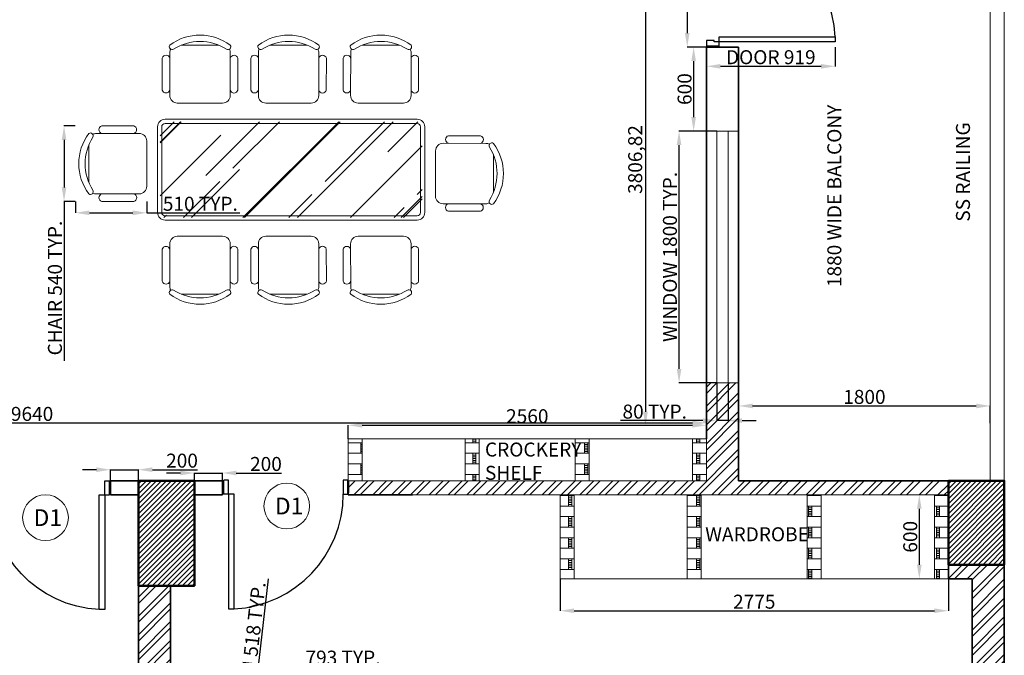
# Model space of a CAD drawing. Units: millimetres. Extents: x -3326 to 29338, y -16792 to 6002.
# Tile 18 of 21: x 22244 to 29282, y -7931 to -3388. Entities that reach past the tile are written whole.
import ezdxf

# ---------------------------------------------------------------- set-up
doc = ezdxf.new("R2010")
doc.units = ezdxf.units.MM
doc.header["$PDMODE"] = 35
doc.header["$PDSIZE"] = 5
for name, color, linetype, lineweight in [('A-ANNO-DIMS', 2, 'Continuous', 13), ('A-ANNO-SYMB', 7, 'Continuous', 18), ('A-AREA-IDEN', 7, 'Continuous', 18), ('A-COLS', 1, 'Continuous', 50), ('A-COLS-PATT', 251, 'Continuous', 13), ('A-DOOR', 3, 'Continuous', 25), ('A-FLOR-CASE', 30, 'Continuous', 18), ('A-FLOR-CASE-PATT', 252, 'Continuous', 13), ('A-FLOR-RAIL', 8, 'Continuous', 20), ('A-FURN-PATT', 252, 'Continuous', 13), ('A-GLAZ', 4, 'Continuous', 18), ('A-WALL', 7, 'Continuous', 35), ('A-WALL-PATT', 252, 'Continuous', 13), ('furn', 28, 'Continuous', 18), ('txt', 7, 'Continuous', 18)]:
    doc.layers.add(name, color=color, linetype=linetype, lineweight=lineweight)
doc.styles.get("Standard").update_dxf_attribs({"font": 'arial.ttf'})
doc.dimstyles.new('ISO-25', dxfattribs={"dimtxt": 100, "dimasz": 100, "dimexe": 1.25, "dimexo": 0.625, "dimtad": 1, "dimtxsty": 'Standard', "dimcen": 2.5, "dimadec": 0, "dimazin": 0, "dimtfac": 1, "dimtmove": 0, "dimatfit": 3, "dimfxl": 1, "dimarcsym": 0})
pattern_1 = [(0, (-10476.645, 1e-12), (0, 75.438), []), (90, (-10270.9, 1e-12), (-114.3, 75.438), [75.438, -75.438]), (90, (-10293.77, 1e-12), (-114.3, 75.438), [75.438, -75.438]), (0, (-10270.905, 12.57), (114.3, 75.438), [-205.74, 22.86]), (0, (-10270.905, 25.146), (114.3, 75.438), [-205.74, 22.86]), (0, (-10270.905, 37.72), (114.3, 75.438), [-205.74, 22.86]), (0, (-10270.905, 50.29), (114.3, 75.438), [-205.74, 22.86]), (0, (-10270.905, 62.865), (114.3, 75.438), [-205.74, 22.86])]
pattern_2 = [(45, (-10476.65, 1e-12), (-67.35192, 67.35192), []), (45, (-10431.74, 1e-12), (-67.35192, 67.35192), [])]

# ---------------------------------------------------------------- blocks, each defined once
blk = doc.blocks.new('A$C13FC179C')
for points in [[(993.9, 100), (920, 100), (920, 1020), (960, 1020), (960, 100), (960, 60), (947.8, 60), (947.8, 0), (993.9, 0)], [(6.1, 0), (46.1, 0), (46.1, 60), (33.9, 60), (33.9, 100), (6.1, 100)], [(6.1, 100), (6.1, 0)], [(993.9, 100), (993.9, 0)]]:
    blk.add_lwpolyline(points)
for points in [[(0, 10), (6.1, 10), (6.1, 90), (0, 90)], [(993.9, 10), (1000, 10), (1000, 90), (993.9, 90)]]:
    blk.add_lwpolyline(points, close=True)
blk.add_arc((960, 100), 920.9, 92.48955, 180)
blk = doc.blocks.new('A$C0CE462CD')
for p, q in [((860, 100), (860, 0)), ((860, 0), (893.9, 0))]:
    blk.add_line(p, q)
for points in [[(860, 100), (860, 920), (818.4, 920), (818.4, 100)], [(0, 10), (6.1, 10), (6.1, 90), (0, 90)], [(893.9, 10), (900, 10), (900, 90), (893.9, 90)]]:
    blk.add_lwpolyline(points, close=True)
for points in [[(6.1, 0), (40, 0), (40, 100), (6.1, 100)], [(6.1, 100), (6.1, 0)], [(860, 100), (893.9, 100), (893.9, 0)]]:
    blk.add_lwpolyline(points)
blk.add_arc((859.1, 101.9), 819.1, 92.8508, 180.13091)
blk = doc.blocks.new('*D16')
at = {"layer": 'A-ANNO-DIMS', "color": 0, "lineweight": -2, "transparency": 16777216}
for p, q in [((26107.3, -7384.6), (26107.3, -7613.9)), ((28882.3, -7384.6), (28882.3, -7613.9)), ((26207.3, -7612.7), (28782.3, -7612.7))]:
    blk.add_line(p, q, dxfattribs=at)
at = {"layer": 'A-ANNO-DIMS', "color": 0, "transparency": 16777216}
for points in [[(26207.3, -7596), (26207.3, -7629.3), (26107.3, -7612.7)], [(28782.3, -7596), (28782.3, -7629.3), (28882.3, -7612.7)]]:
    blk.add_solid(points, dxfattribs=at)
at = {"layer": 'Defpoints', "color": 0, "transparency": 16777216}
for p in [(26107.3, -7384), (28882.3, -7384), (28882.3, -7612.7)]:
    blk.add_point(p, dxfattribs=at)
at = {"layer": 'A-ANNO-DIMS', "color": 0, "transparency": 16777216, "insert": (27494.8, -7561), "char_height": 100, "attachment_point": 5}
blk.add_mtext('2775', dxfattribs=at)
blk = doc.blocks.new('*D31')
at = {"layer": 'A-ANNO-DIMS', "color": 0, "lineweight": -2, "transparency": 16777216}
for p, q in [((22792.3, -6604.5), (22692.3, -6604.5)), ((22892.3, -6683.3), (22892.3, -6603.3)), ((22892.3, -6604.5), (23092.3, -6604.5)), ((23092.3, -6683.3), (23092.3, -6603.3)), ((23192.3, -6604.5), (23515.9, -6604.5))]:
    blk.add_line(p, q, dxfattribs=at)
at = {"layer": 'A-ANNO-DIMS', "color": 0, "transparency": 16777216}
for points in [[(22792.3, -6587.8), (22792.3, -6621.2), (22892.3, -6604.5)], [(23192.3, -6587.8), (23192.3, -6621.2), (23092.3, -6604.5)]]:
    blk.add_solid(points, dxfattribs=at)
at = {"layer": 'Defpoints', "color": 0, "transparency": 16777216}
for p in [(23092.3, -6604.5), (22892.3, -6684), (23092.3, -6684)]:
    blk.add_point(p, dxfattribs=at)
at = {"layer": 'A-ANNO-DIMS', "color": 0, "transparency": 16777216, "insert": (23404.1, -6552.8), "char_height": 100, "attachment_point": 5}
blk.add_mtext('200', dxfattribs=at)
blk = doc.blocks.new('*D32')
at = {"layer": 'A-ANNO-DIMS', "color": 0, "lineweight": -2, "transparency": 16777216}
for p, q in [((23392.3, -6628.3), (23292.3, -6628.3)), ((23492.3, -6683.3), (23492.3, -6627)), ((23492.3, -6628.3), (23692.3, -6628.3)), ((23692.3, -6683.3), (23692.3, -6627)), ((23792.3, -6628.3), (24115.9, -6628.3))]:
    blk.add_line(p, q, dxfattribs=at)
at = {"layer": 'A-ANNO-DIMS', "color": 0, "transparency": 16777216}
for points in [[(23392.3, -6611.6), (23392.3, -6644.9), (23492.3, -6628.3)], [(23792.3, -6611.6), (23792.3, -6644.9), (23692.3, -6628.3)]]:
    blk.add_solid(points, dxfattribs=at)
at = {"layer": 'Defpoints', "color": 0, "transparency": 16777216}
for p in [(23492.3, -6684), (23692.3, -6628.3), (23692.3, -6684)]:
    blk.add_point(p, dxfattribs=at)
at = {"layer": 'A-ANNO-DIMS', "color": 0, "transparency": 16777216, "insert": (24004.1, -6576.6), "char_height": 100, "attachment_point": 5}
blk.add_mtext('200', dxfattribs=at)
blk = doc.blocks.new('*D33')
at = {"layer": 'A-ANNO-DIMS', "color": 0, "lineweight": -2, "transparency": 16777216}
for p, q in [((24592.3, -6383.3), (24592.3, -6285.8)), ((24692.3, -6287), (27052.3, -6287)), ((27152.3, -6383.3), (27152.3, -6285.8))]:
    blk.add_line(p, q, dxfattribs=at)
at = {"layer": 'A-ANNO-DIMS', "color": 0, "transparency": 16777216}
for points in [[(24692.3, -6270.4), (24692.3, -6303.7), (24592.3, -6287)], [(27052.3, -6270.4), (27052.3, -6303.7), (27152.3, -6287)]]:
    blk.add_solid(points, dxfattribs=at)
at = {"layer": 'Defpoints', "color": 0, "transparency": 16777216}
for p in [(27152.3, -6287), (24592.3, -6384), (27152.3, -6384)]:
    blk.add_point(p, dxfattribs=at)
at = {"layer": 'A-ANNO-DIMS', "color": 0, "transparency": 16777216, "insert": (25872.3, -6235.3), "char_height": 100, "attachment_point": 5}
blk.add_mtext('2560', dxfattribs=at)
blk = doc.blocks.new('*D83')
at = {"layer": 'A-ANNO-DIMS', "color": 0, "lineweight": -2, "transparency": 16777216}
for p, q in [((28675.2, -6784), (28675.9, -6784)), ((28674.6, -6884), (28674.6, -7284)), ((28675.2, -7384), (28675.9, -7384))]:
    blk.add_line(p, q, dxfattribs=at)
at = {"layer": 'A-ANNO-DIMS', "color": 0, "transparency": 16777216}
for points in [[(28657.9, -6884), (28691.3, -6884), (28674.6, -6784)], [(28657.9, -7284), (28691.3, -7284), (28674.6, -7384)]]:
    blk.add_solid(points, dxfattribs=at)
at = {"layer": 'Defpoints', "color": 0, "transparency": 16777216}
for p in [(28674.6, -6784), (28674.6, -7384), (28674.6, -7384)]:
    blk.add_point(p, dxfattribs=at)
at = {"layer": 'A-ANNO-DIMS', "color": 0, "transparency": 16777216, "insert": (28622.9, -7084), "char_height": 100, "attachment_point": 5, "rotation": 90}
blk.add_mtext('600', dxfattribs=at)
blk = doc.blocks.new('*D93')
at = {"layer": 'A-ANNO-DIMS', "color": 0, "lineweight": -2, "transparency": 16777216}
for p, q in [((27382.3, -6273.2), (27382.3, -6147.7)), ((27482.3, -6148.9), (29082.3, -6148.9)), ((29182.3, -6273.2), (29182.3, -6147.7))]:
    blk.add_line(p, q, dxfattribs=at)
at = {"layer": 'A-ANNO-DIMS', "color": 0, "transparency": 16777216}
for points in [[(27482.3, -6132.3), (27482.3, -6165.6), (27382.3, -6148.9)], [(29082.3, -6132.3), (29082.3, -6165.6), (29182.3, -6148.9)]]:
    blk.add_solid(points, dxfattribs=at)
at = {"layer": 'Defpoints', "color": 0, "transparency": 16777216}
for p in [(29182.3, -6148.9), (27382.3, -6273.8), (29182.3, -6273.8)]:
    blk.add_point(p, dxfattribs=at)
at = {"layer": 'A-ANNO-DIMS', "color": 0, "transparency": 16777216, "insert": (28282.3, -6097.3), "char_height": 100, "attachment_point": 5}
blk.add_mtext('1800', dxfattribs=at)
blk = doc.blocks.new('*D94')
at = {"layer": 'A-ANNO-DIMS', "color": 0, "lineweight": -2, "transparency": 16777216}
for p, q in [((27151.7, -3584), (27060.1, -3584)), ((27061.4, -3684), (27061.4, -4084)), ((27151.7, -4184), (27060.1, -4184))]:
    blk.add_line(p, q, dxfattribs=at)
at = {"layer": 'A-ANNO-DIMS', "color": 0, "transparency": 16777216}
for points in [[(27044.7, -3684), (27078.1, -3684), (27061.4, -3584)], [(27044.7, -4084), (27078.1, -4084), (27061.4, -4184)]]:
    blk.add_solid(points, dxfattribs=at)
at = {"layer": 'Defpoints', "color": 0, "transparency": 16777216}
for p in [(27152.3, -3584), (27061.4, -4184), (27152.3, -4184)]:
    blk.add_point(p, dxfattribs=at)
at = {"layer": 'A-ANNO-DIMS', "color": 0, "transparency": 16777216, "insert": (27009.7, -3884), "char_height": 100, "attachment_point": 5, "rotation": 90}
blk.add_mtext('600', dxfattribs=at)
blk = doc.blocks.new('*D96')
at = {"layer": 'A-ANNO-DIMS', "color": 0, "lineweight": -2, "transparency": 16777216}
for p, q in [((26717.8, -2484), (26718.5, -2484)), ((26717.2, -2584), (26717.2, -6190.8)), ((26717.8, -6290.8), (26718.5, -6290.8))]:
    blk.add_line(p, q, dxfattribs=at)
at = {"layer": 'A-ANNO-DIMS', "color": 0, "transparency": 16777216}
for points in [[(26700.5, -2584), (26733.9, -2584), (26717.2, -2484)], [(26700.5, -6190.8), (26733.9, -6190.8), (26717.2, -6290.8)]]:
    blk.add_solid(points, dxfattribs=at)
at = {"layer": 'Defpoints', "color": 0, "transparency": 16777216}
for p in [(26717.2, -2484), (26717.2, -6290.8), (26717.2, -6290.8)]:
    blk.add_point(p, dxfattribs=at)
at = {"layer": 'A-ANNO-DIMS', "color": 0, "transparency": 16777216, "insert": (26656.5, -4387.4), "char_height": 100, "attachment_point": 5, "rotation": 90}
blk.add_mtext('3806,82', dxfattribs=at)
blk = doc.blocks.new('*D97')
at = {"layer": 'A-ANNO-DIMS', "color": 0, "lineweight": -2, "transparency": 16777216}
for p, q in [((27152.3, -6119.9), (27152.3, -6271.6)), ((17512.3, -6265.8), (17512.3, -6271.6)), ((17612.3, -6270.4), (27052.3, -6270.4))]:
    blk.add_line(p, q, dxfattribs=at)
at = {"layer": 'A-ANNO-DIMS', "color": 0, "transparency": 16777216}
for points in [[(17612.3, -6253.7), (17612.3, -6287), (17512.3, -6270.4)], [(27052.3, -6253.7), (27052.3, -6287), (27152.3, -6270.4)]]:
    blk.add_solid(points, dxfattribs=at)
at = {"layer": 'Defpoints', "color": 0, "transparency": 16777216}
for p in [(27152.3, -6119.3), (17512.3, -6265.2), (27152.3, -6270.4)]:
    blk.add_point(p, dxfattribs=at)
at = {"layer": 'A-ANNO-DIMS', "color": 0, "transparency": 16777216, "insert": (22332.3, -6218.7), "char_height": 100, "attachment_point": 5}
blk.add_mtext('9640', dxfattribs=at)
blk = doc.blocks.new('CHAIR-DINING')
for p, q in [((54.3, 125.8), (54, 431.8)), ((107.9, 485.8), (431.9, 486.2)), ((486, 432.2), (486.3, 126.2)), ((0, 393.5), (0.2, 164)), ((540, 394), (540.2, 164.5)), ((404.2, 72.1), (136.4, 71.9))]:
    blk.add_line(p, q)
for centre, radius, start, end in [((108, 431.8), 54, 90.0573, 180.0573), ((432, 432.2), 54, 0.0573, 90.0573), ((27, 385.6), 28.1, 16.3175, 163.79709), ((513, 386.1), 28.1, 16.3175, 163.79709), ((27.2, 171.9), 28.1, 196.3175, 343.79709), ((513.2, 172.4), 28.1, 196.3175, 343.79709), ((70.1, 83.6), 19.7, 58.02988, 216.74736), ((108.3, 125.8), 54, 180.0573, 207.64174), ((270, 360), 360, 233.1874, 306.92719), ((270, 399.2), 353.5, 237.63305, 302.48154), ((470.5, 84), 19.7, 323.36723, 122.08471), ((432.3, 126.2), 54, 332.47286, 0.0573)]:
    blk.add_arc(centre, radius, start, end)
blk = doc.blocks.new('TAG-D1')
blk.add_circle((163.3, 163.3), 163.3)
at = {"insert": (78, 223.5), "char_height": 120, "attachment_point": 1}
blk.add_mtext_dynamic_manual_height_columns('D1', width=137.943, gutter_width=12.5, heights=[0], dxfattribs=at)
blk = doc.blocks.new('GLAZ-1800x80')
for p, q in [((0, 80), (1800, 80)), ((0, 0), (1800, 0))]:
    blk.add_line(p, q)
blk = doc.blocks.new('*D190')
at = {"layer": 'A-ANNO-DIMS', "color": 0, "lineweight": -2, "transparency": 16777216}
for p, q in [((24158.2, -8133.6), (24158.2, -8011.3)), ((24258.2, -8012.6), (24851.6, -8012.6)), ((24951.6, -8133.6), (24951.6, -8011.3))]:
    blk.add_line(p, q, dxfattribs=at)
at = {"layer": 'A-ANNO-DIMS', "color": 0, "transparency": 16777216}
for points in [[(24258.2, -7995.9), (24258.2, -8029.2), (24158.2, -8012.6)], [(24851.6, -7995.9), (24851.6, -8029.2), (24951.6, -8012.6)]]:
    blk.add_solid(points, dxfattribs=at)
at = {"layer": 'Defpoints', "color": 0, "transparency": 16777216}
for p in [(24951.6, -8012.6), (24158.2, -8134.2), (24951.6, -8134.2)]:
    blk.add_point(p, dxfattribs=at)
at = {"layer": 'A-ANNO-DIMS', "color": 0, "transparency": 16777216, "insert": (24554.9, -7960.9), "char_height": 100, "attachment_point": 5}
blk.add_mtext('793 TYP.', dxfattribs=at)
blk = doc.blocks.new('*D201')
at = {"layer": 'A-ANNO-DIMS', "color": 0, "lineweight": -2, "transparency": 16777216}
for p, q in [((27153.3, -3584), (27153.3, -3722.5)), ((28072.8, -3584), (28072.8, -3722.5)), ((27253.3, -3721.3), (27972.8, -3721.3))]:
    blk.add_line(p, q, dxfattribs=at)
at = {"layer": 'A-ANNO-DIMS', "color": 0, "transparency": 16777216}
for points in [[(27253.3, -3704.6), (27253.3, -3737.9), (27153.3, -3721.3)], [(27972.8, -3704.6), (27972.8, -3737.9), (28072.8, -3721.3)]]:
    blk.add_solid(points, dxfattribs=at)
at = {"layer": 'Defpoints', "color": 0, "transparency": 16777216}
for p in [(27153.3, -3583.3), (28072.8, -3583.3), (28072.8, -3721.3)]:
    blk.add_point(p, dxfattribs=at)
at = {"layer": 'A-ANNO-DIMS', "color": 0, "transparency": 16777216, "insert": (27613.1, -3668.9), "char_height": 100, "attachment_point": 5}
blk.add_mtext('DOOR 919', dxfattribs=at)
blk = doc.blocks.new('*D202')
at = {"layer": 'A-ANNO-DIMS', "color": 0, "lineweight": -2, "transparency": 16777216}
for p, q in [((27152.7, -2681.9), (27014.2, -2681.9)), ((27015.4, -2781.9), (27015.4, -3483.3)), ((27152.7, -3583.3), (27014.2, -3583.3))]:
    blk.add_line(p, q, dxfattribs=at)
at = {"layer": 'A-ANNO-DIMS', "color": 0, "transparency": 16777216}
for points in [[(26998.8, -2781.9), (27032.1, -2781.9), (27015.4, -2681.9)], [(26998.8, -3483.3), (27032.1, -3483.3), (27015.4, -3583.3)]]:
    blk.add_solid(points, dxfattribs=at)
at = {"layer": 'Defpoints', "color": 0, "transparency": 16777216}
for p in [(27153.3, -2681.9), (27015.4, -3583.3), (27153.3, -3583.3)]:
    blk.add_point(p, dxfattribs=at)
at = {"layer": 'A-ANNO-DIMS', "color": 0, "transparency": 16777216, "insert": (26963.7, -3132.6), "char_height": 100, "attachment_point": 5, "rotation": 90}
blk.add_mtext('901', dxfattribs=at)
blk = doc.blocks.new('*D203')
at = {"layer": 'A-ANNO-DIMS', "color": 0, "lineweight": -2, "transparency": 16777216}
for p, q in [((27226.7, -4184), (26956.1, -4184)), ((26957.3, -5884), (26957.3, -4284)), ((27226.7, -5984), (26956.1, -5984))]:
    blk.add_line(p, q, dxfattribs=at)
at = {"layer": 'A-ANNO-DIMS', "color": 0, "transparency": 16777216}
for points in [[(26940.6, -4284), (26974, -4284), (26957.3, -4184)], [(26940.6, -5884), (26974, -5884), (26957.3, -5984)]]:
    blk.add_solid(points, dxfattribs=at)
at = {"layer": 'Defpoints', "color": 0, "transparency": 16777216}
for p in [(26957.3, -4184), (27227.3, -4184), (27227.3, -5984)]:
    blk.add_point(p, dxfattribs=at)
at = {"layer": 'A-ANNO-DIMS', "color": 0, "transparency": 16777216, "insert": (26904.9, -5084), "char_height": 100, "attachment_point": 5, "rotation": 90}
blk.add_mtext('WINDOW 1800 TYP.', dxfattribs=at)
blk = doc.blocks.new('*D204')
at = {"layer": 'A-ANNO-DIMS', "color": 0, "lineweight": -2, "transparency": 16777216}
for p, q in [((27227.3, -5984.6), (27227.3, -6255.2)), ((27307.3, -5984.6), (27307.3, -6255.2)), ((27127.3, -6254), (26539.1, -6254)), ((27307.3, -6254), (27227.3, -6254)), ((27407.3, -6254), (27507.3, -6254))]:
    blk.add_line(p, q, dxfattribs=at)
at = {"layer": 'A-ANNO-DIMS', "color": 0, "transparency": 16777216}
for points in [[(27127.3, -6237.3), (27127.3, -6270.6), (27227.3, -6254)], [(27407.3, -6237.3), (27407.3, -6270.6), (27307.3, -6254)]]:
    blk.add_solid(points, dxfattribs=at)
at = {"layer": 'Defpoints', "color": 0, "transparency": 16777216}
for p in [(27227.3, -5984), (27307.3, -5984), (27227.3, -6254)]:
    blk.add_point(p, dxfattribs=at)
at = {"layer": 'A-ANNO-DIMS', "color": 0, "transparency": 16777216, "insert": (26783.2, -6202.3), "char_height": 100, "attachment_point": 5}
blk.add_mtext('80 TYP.', dxfattribs=at)
blk = doc.blocks.new('*D211')
at = {"layer": 'A-ANNO-DIMS', "color": 0, "lineweight": -2, "transparency": 16777216}
for p, q in [((22641.2, -4147.1), (22559.6, -4147.1)), ((22560.8, -4247.1), (22560.8, -4587.3)), ((22641.2, -4687.3), (22559.6, -4687.3)), ((22560.8, -4687.3), (22560.8, -5825.4))]:
    blk.add_line(p, q, dxfattribs=at)
at = {"layer": 'A-ANNO-DIMS', "color": 0, "transparency": 16777216}
for points in [[(22544.2, -4247.1), (22577.5, -4247.1), (22560.8, -4147.1)], [(22544.2, -4587.3), (22577.5, -4587.3), (22560.8, -4687.3)]]:
    blk.add_solid(points, dxfattribs=at)
at = {"layer": 'Defpoints', "color": 0, "transparency": 16777216}
for p in [(22641.9, -4147.1), (22560.8, -4687.3), (22641.9, -4687.3)]:
    blk.add_point(p, dxfattribs=at)
at = {"layer": 'A-ANNO-DIMS', "color": 0, "transparency": 16777216, "insert": (22508.5, -5306.4), "char_height": 100, "attachment_point": 5, "rotation": 90}
blk.add_mtext('CHAIR 540 TYP.', dxfattribs=at)
blk = doc.blocks.new('*D212')
at = {"layer": 'A-ANNO-DIMS', "color": 0, "lineweight": -2, "transparency": 16777216}
for p, q in [((22641.9, -4688), (22641.9, -4769.6)), ((23152.1, -4688), (23152.1, -4769.6)), ((22741.9, -4768.4), (23052.1, -4768.4)), ((23152.1, -4768.4), (23817.8, -4768.4))]:
    blk.add_line(p, q, dxfattribs=at)
at = {"layer": 'A-ANNO-DIMS', "color": 0, "transparency": 16777216}
for points in [[(22741.9, -4751.7), (22741.9, -4785), (22641.9, -4768.4)], [(23052.1, -4751.7), (23052.1, -4785), (23152.1, -4768.4)]]:
    blk.add_solid(points, dxfattribs=at)
at = {"layer": 'Defpoints', "color": 0, "transparency": 16777216}
for p in [(22641.9, -4687.3), (23152.1, -4687.3), (23152.1, -4768.4)]:
    blk.add_point(p, dxfattribs=at)
at = {"layer": 'A-ANNO-DIMS', "color": 0, "transparency": 16777216, "insert": (23535, -4716.7), "char_height": 100, "attachment_point": 5}
blk.add_mtext('510 TYP.', dxfattribs=at)
blk = doc.blocks.new('*D215')
at = {"layer": 'A-ANNO-DIMS', "color": 0, "lineweight": -2, "transparency": 16777216}
for p, q in [((23896.1, -8496.3), (24021.7, -7384)), ((23819.5, -8487.6), (23897.4, -8496.4)), ((23849.2, -8911.8), (23884.9, -8595.6)), ((23761.4, -9002.6), (23839.2, -9011.3))]:
    blk.add_line(p, q, dxfattribs=at)
at = {"layer": 'A-ANNO-DIMS', "color": 0, "transparency": 16777216}
for points in [[(23868.3, -8593.8), (23901.5, -8597.5), (23896.1, -8496.3)], [(23832.6, -8910), (23865.8, -8913.7), (23838, -9011.2)]]:
    blk.add_solid(points, dxfattribs=at)
at = {"layer": 'Defpoints', "color": 0, "transparency": 16777216}
for p in [(23818.9, -8487.6), (23896.1, -8496.3), (23760.8, -9002.5)]:
    blk.add_point(p, dxfattribs=at)
at = {"layer": 'A-ANNO-DIMS', "color": 0, "transparency": 16777216, "insert": (23912.5, -7884.6), "char_height": 100, "attachment_point": 5, "rotation": 83.55971}
blk.add_mtext('BASIN 518 TYP.', dxfattribs=at)

msp = doc.modelspace()

# ---------------------------------------------------------------- hatches: boundary and pattern name
at = {"layer": 'A-COLS-PATT'}
h = msp.add_hatch(dxfattribs=at)
h.set_pattern_fill('ANSI31', color=256, scale=8)
h.set_pattern_definition([(45, (-18946.33, 3485.585), (-17.960512, 17.960512), [])])
h.paths.add_polyline_path([(23492.301, -6683.952), (23092.301, -6683.952), (23092.301, -7433.952), (23492.301, -7433.952)])
h = msp.add_hatch(dxfattribs=at)
h.set_pattern_fill('ANSI31', color=256, scale=8)
h.set_pattern_definition([(45, (-12839, -76.948), (-17.960512, 17.960512), [])])
h.paths.add_polyline_path([(28882.301, -7283.952), (29282.301, -7283.952), (29282.301, -6683.952), (28882.301, -6683.952)])
at = {"layer": 'A-FLOR-CASE-PATT'}
h = msp.add_hatch(dxfattribs=at)
h.set_pattern_fill('BRSTONE', color=256, scale=9)
h.set_pattern_definition(pattern_1)
h.paths.add_polyline_path([(24692.301, -6383.952), (24592.301, -6383.952), (24592.301, -6683.952), (24692.301, -6683.952)])
h.paths.add_polyline_path([(25528.967, -6383.952), (25428.967, -6383.952), (25428.967, -6683.952), (25528.967, -6683.952)])
h.paths.add_polyline_path([(26315.634, -6383.952), (26215.634, -6383.952), (26215.634, -6683.952), (26315.634, -6683.952)])
h.paths.add_polyline_path([(27152.301, -6383.952), (27052.301, -6383.952), (27052.301, -6683.952), (27152.301, -6683.952)])
h = msp.add_hatch(dxfattribs=at)
h.set_pattern_fill('BRSTONE', color=256, scale=9)
h.set_pattern_definition(pattern_1)
h.paths.add_polyline_path([(26207.301, -6783.952), (26107.301, -6783.952), (26107.301, -7383.952), (26207.301, -7383.952)])
h.paths.add_polyline_path([(27115.634, -6783.952), (27015.634, -6783.952), (27015.634, -7383.952), (27115.634, -7383.952)])
h.paths.add_polyline_path([(27873.967, -7383.952), (27973.967, -7383.952), (27973.967, -6783.952), (27873.967, -6783.952)])
h.paths.add_polyline_path([(28782.301, -7383.952), (28882.301, -7383.952), (28882.301, -7283.952), (28882.301, -6783.952), (28782.301, -6783.952)])
h.paths.add_polyline_path([(27117.498, -7172.598), (27990.213, -7172.598), (27990.213, -6966.527), (27117.498, -6966.527)], flags=9)
at = {"layer": 'A-FURN-PATT'}
h = msp.add_hatch(dxfattribs=at)
h.set_pattern_fill('AR-RROOF', color=256, scale=400, angle=-135, style=0)
h.set_pattern_definition([(225, (64133.74, 17389.84), (-339.4113, -905.0967), [6000, -800, 2000, -400]), (225, (63899, 16872.24), (659.0235, -93.338), [1200, -132, 2400, -300]), (225, (64232.74, 17008), (-1281.2775, -1660.2867), [3200, -560, 1600, -400])])
edge = h.paths.add_edge_path()
edge.add_line((25121.037, -4765.986), (25121.037, -4153.986))
edge.add_arc((25085.037, -4153.986), 36, 0, 90)
edge.add_line((25085.037, -4117.986), (23283.037, -4117.986))
edge.add_arc((23283.037, -4153.986), 36, 90, 180)
edge.add_line((23247.037, -4153.986), (23247.037, -4765.986))
edge.add_arc((23283.037, -4765.986), 36, -180, -90)
edge.add_line((23283.037, -4801.986), (25085.037, -4801.986))
edge.add_arc((25085.037, -4765.986), 36, -90, 0)
at = {"layer": 'A-WALL-PATT'}
h = msp.add_hatch(dxfattribs=at)
h.set_pattern_fill('ANSI32', color=256, scale=10)
h.set_pattern_definition(pattern_2)
h.paths.add_polyline_path([(29282.301, -7283.952), (28882.301, -7283.952), (28882.301, -7383.952), (29052.301, -7383.952), (29052.301, -10763.952), (29282.301, -10763.952)])
h.paths.add_polyline_path([(29282.301, -11263.952), (29052.301, -11263.952), (29052.301, -12763.952), (29282.301, -12763.952)])
h.paths.add_polyline_path([(25052.301, -11263.952), (25652.301, -11263.952), (25652.301, -11123.904), (25652.289, -11123.904), (25652.289, -11033.952), (25052.301, -11033.952), (24572.301, -11033.952), (24572.301, -11263.952), (24822.301, -11263.952), (24822.301, -12763.952), (25052.301, -12763.952)])
h.paths.add_polyline_path([(26902.301, -11033.952), (26552.301, -11033.952), (26552.301, -11263.952), (26902.301, -11263.952)])
h.paths.add_polyline_path([(21992.301, -6683.952), (21362.301, -6683.952), (17512.301, -6683.952), (17512.301, -6783.952), (21362.301, -6783.952), (21992.301, -6783.952)])
h.paths.add_polyline_path([(17512.301, -7283.952), (17282.301, -7283.952), (17282.301, -12163.952), (17512.301, -12163.952), (17512.301, -11263.952), (18112.301, -11263.952), (18112.301, -11033.952), (17512.301, -11033.952)])
h.paths.add_polyline_path([(21462.301, -8211.864), (21462.064, -8211.864), (21462.064, -8142.609), (21462.301, -8133.952), (21362.301, -8133.952), (21362.301, -8233.952), (21362.301, -11033.952), (21162.301, -11033.952), (21162.301, -11263.952), (21362.301, -11263.952), (21362.301, -12763.952), (21592.301, -12763.952), (21592.301, -11263.952), (21992.301, -11263.952), (21992.301, -11033.952), (21592.301, -11033.952), (21462.301, -11033.952)])
h.paths.add_polyline_path([(24152.301, -8133.952), (23322.301, -8133.952), (23322.301, -7433.952), (23092.301, -7433.952), (23092.301, -8133.952), (22241.021, -8133.952), (22241.021, -8142.609), (22241.182, -8142.609), (22241.182, -8211.864), (22241.021, -8233.952), (23092.301, -8233.952), (23092.301, -10513.206), (23322.301, -10513.206), (23322.301, -8233.952), (24152.301, -8233.952)])
h.paths.add_polyline_path([(25052.301, -8233.952), (25052.301, -8133.952), (24952.301, -8133.952), (24952.301, -11033.952), (25052.301, -11033.952)])
h.paths.add_polyline_path([(23972.301, -11033.952), (23493.251, -11033.952), (23493.251, -11263.952), (23972.301, -11263.952)])
h.paths.add_polyline_path([(23092.301, -11033.952), (22592.301, -11033.952), (22592.301, -11263.952), (23092.301, -11263.952)])
h.paths.add_polyline_path([(28882.301, -11033.952), (28702.301, -11033.952), (28702.301, -11263.952), (28882.301, -11263.952)])
h.paths.add_polyline_path([(17512.301, -3883.952), (17387.589, -3883.952), (17387.589, -3888.07), (17282.301, -3888.07), (17282.301, -6683.952), (17512.301, -6683.952)])
h.paths.add_polyline_path([(21462.301, -2183.952), (21362.301, -2183.952), (21362.301, -2383.952), (17282.301, -2383.952), (17282.301, -2483.952), (17512.301, -2483.952), (21462.301, -2483.952)])
h.paths.add_polyline_path([(17512.301, -2483.952), (17282.301, -2483.952), (17282.301, -2833.952), (17512.301, -2833.952)])
h.paths.add_polyline_path([(21462.301, 1866.048), (21992.301, 1866.048), (21992.301, 2096.048), (21592.301, 2096.048), (21592.301, 3596.048), (21362.301, 3596.048), (21362.301, 1866.048), (21362.301, -1283.952), (21462.301, -1283.952)])
h.paths.add_polyline_path([(17512.301, 1496.048), (17282.301, 1496.048), (17282.301, -1983.952), (17612.301, -1983.952), (17612.301, -1883.952), (17512.301, -1883.952)])
h.paths.add_polyline_path([(17512.301, 3596.048), (17282.301, 3596.048), (17282.301, 2096.048), (17512.301, 2096.048)])
h.paths.add_polyline_path([(18135.023, 2096.048), (17685.023, 2096.048), (17685.023, 1866.048), (18135.023, 1866.048), (18135.023, 1876.048), (18128.942, 1876.048), (18128.942, 1956.048), (18135.023, 1956.048)])
h.paths.add_polyline_path([(19385.023, 2096.048), (19035.023, 2096.048), (19035.023, 1866.048), (19385.023, 1866.048)])
h.paths.add_polyline_path([(21362.301, 2096.048), (21185.023, 2096.048), (21185.023, 1866.048), (21362.301, 1866.048)])
h.paths.add_polyline_path([(23092.301, 2096.048), (22592.301, 2096.048), (22592.301, 1866.048), (23092.301, 1866.048)])
h.paths.add_polyline_path([(23972.301, 2096.048), (23492.301, 2096.048), (23492.301, 1866.048), (23972.301, 1866.048)])
h.paths.add_polyline_path([(23972.301, 2496.048), (23872.301, 2496.048), (23872.301, 2096.048), (23972.301, 2096.048)])
h.paths.add_polyline_path([(22692.301, 2496.048), (22592.301, 2496.048), (22592.301, 2096.048), (22692.301, 2096.048)])
h.paths.add_polyline_path([(23322.301, 1346.048), (23092.301, 1346.048), (23092.301, -1733.952), (23322.301, -1733.952)])
h.paths.add_polyline_path([(23092.301, -933.952), (22262.301, -933.952), (22262.301, -1033.952), (23092.301, -1033.952)])
h.paths.add_polyline_path([(24952.301, -1433.952), (24952.301, -1733.952), (23492.301, -1733.952), (23492.301, -1833.952), (24952.301, -1833.952), (24952.301, -2483.952), (25052.301, -2483.952), (25052.301, -2466.23), (25049.26, -2466.23), (25049.26, -2386.23), (25049.941, -1433.952)])
h.paths.add_polyline_path([(22692.301, -11263.952), (22592.301, -11263.952), (22592.301, -11663.952), (22692.301, -11663.952)])
h.paths.add_polyline_path([(23972.301, -11263.952), (23872.301, -11263.952), (23872.301, -11663.952), (23972.301, -11663.952)])
h = msp.add_hatch(dxfattribs=at)
h.set_pattern_fill('ANSI32', color=256, scale=10)
h.set_pattern_definition(pattern_2)
h.paths.add_polyline_path([(27382.301, -5983.952), (27152.301, -5983.952), (27152.301, -6383.952), (27152.301, -6683.952), (25428.967, -6683.952), (25428.967, -6783.952), (28882.301, -6783.952), (28882.301, -6683.952), (27382.301, -6683.952)])
h.paths.add_polyline_path([(25428.967, -6683.952), (25052.301, -6683.952), (24592.301, -6683.952), (24592.301, -6783.952), (25052.301, -6783.952), (25428.967, -6783.952)])

# ---------------------------------------------------------------- linework, layer by layer
at = {"layer": 'A-COLS'}
for points in [[(23092.301, -6683.952), (23492.301, -6683.952), (23492.301, -7433.952), (23092.301, -7433.952)], [(28882.301, -6683.952), (29282.301, -6683.952), (29282.301, -7283.952), (28882.301, -7283.952)]]:
    msp.add_lwpolyline(points, close=True, dxfattribs=at)
at = {"layer": 'A-FLOR-CASE'}
for p, q in [((24592.301, -6683.952), (24592.301, -6383.952)), ((24592.301, -6383.952), (24692.301, -6383.952)), ((24692.301, -6683.952), (24692.301, -6383.952)), ((24692.301, -6383.952), (27052.301, -6383.952)), ((25428.967, -6383.952), (25428.967, -6683.952)), ((25528.967, -6383.952), (25528.967, -6683.952)), ((26215.634, -6383.952), (26215.634, -6683.952)), ((26315.634, -6383.952), (26315.634, -6683.952)), ((27052.301, -6383.952), (27052.301, -6683.952)), ((27052.301, -6383.952), (27152.301, -6383.952)), ((27152.301, -6383.952), (27152.301, -6683.952)), ((25052.301, -6683.952), (24592.301, -6683.952)), ((27152.301, -6683.952), (25052.301, -6683.952)), ((28882.301, -6783.952), (25052.301, -6783.952)), ((26107.301, -7383.952), (26107.301, -6783.952)), ((26207.301, -7383.952), (26207.301, -6783.952)), ((27015.634, -7383.952), (27015.634, -6783.952)), ((27115.634, -7383.952), (27115.634, -6783.952)), ((27873.967, -7383.952), (27873.967, -6783.952)), ((27973.967, -7383.952), (27973.967, -6783.952)), ((28782.301, -6783.952), (28782.301, -7383.952)), ((28882.301, -7383.952), (26107.301, -7383.952))]:
    msp.add_line(p, q, dxfattribs=at)
at = {"layer": 'A-FLOR-RAIL'}
for p, q in [((29182.301, -2483.676), (29182.301, -6683.952)), ((29282.301, -2483.676), (29282.301, -6683.952))]:
    msp.add_line(p, q, dxfattribs=at)
at = {"layer": 'A-GLAZ'}
for p, q in [((27382.301, -4183.952), (27152.301, -4183.952)), ((27382.301, -5983.952), (27152.301, -5983.952))]:
    msp.add_line(p, q, dxfattribs=at)
at = {"layer": 'A-WALL'}
for p, q in [((27382.301, -3583.952), (27152.301, -3583.952)), ((27152.301, -3583.952), (27152.301, -6383.952)), ((27382.301, -3583.952), (27382.301, -6683.952)), ((22892.301, -6683.952), (22892.301, -6783.952)), ((23692.301, -6683.952), (22892.301, -6683.952)), ((23092.301, -6683.952), (23092.301, -8133.952)), ((23692.301, -6683.952), (23692.301, -6783.952)), ((24592.301, -6683.952), (24592.301, -6783.952)), ((29052.301, -6683.952), (27382.301, -6683.952)), ((29282.301, -6683.952), (29282.301, -12763.952)), ((23092.301, -6783.952), (22892.301, -6783.952)), ((23692.301, -6783.952), (23492.301, -6783.952)), ((25052.301, -6783.952), (24592.301, -6783.952)), ((28882.301, -7283.952), (28882.301, -7383.952)), ((28882.301, -7383.952), (29052.301, -7383.952)), ((29052.301, -7383.952), (29052.301, -10763.952)), ((23322.301, -7433.952), (23322.301, -8133.952))]:
    msp.add_line(p, q, dxfattribs=at)
at = {"layer": 'furn'}
for points in [[(25139.037, -4765.986), (25139.037, -4153.986, 0.41421356), (25085.037, -4099.986), (23283.037, -4099.986, 0.41421356), (23229.037, -4153.986), (23229.037, -4765.986, 0.41421356), (23283.037, -4819.986), (25085.037, -4819.986, 0.41421356)], [(25109.037, -4765.986), (25109.037, -4153.986, 0.41421356), (25085.037, -4129.986), (23283.037, -4129.986, 0.41421356), (23259.037, -4153.986), (23259.037, -4765.986, 0.41421356), (23283.037, -4789.986), (25085.037, -4789.986, 0.41421356)]]:
    msp.add_lwpolyline(points, format="xyb", close=True, dxfattribs=at)

# ---------------------------------------------------------------- block references
at = {"layer": 'A-ANNO-SYMB'}
for p in [(23989.856, -7027.635), (22264.817, -7110.715)]:
    msp.add_blockref('TAG-D1', p, dxfattribs=at)
at = {"layer": 'A-DOOR', "xscale": 0.9014347414877603, "yscale": 0.9014347414877603, "zscale": 0.9014347414877603, "rotation": 270}
msp.add_blockref('A$C13FC179C', (27153.349, -2681.902), dxfattribs=at)
at = {"layer": 'A-DOOR', "xscale": -1, "rotation": 180}
msp.add_blockref('A$C0CE462CD', (21992.301, -6683.952), dxfattribs=at)
at = {"layer": 'A-DOOR', "rotation": 180}
msp.add_blockref('A$C0CE462CD', (24596.354, -6678.967), dxfattribs=at)
at = {"layer": 'A-GLAZ', "rotation": 90}
msp.add_blockref('GLAZ-1800x80', (27307.301, -5983.952), dxfattribs=at)
at = {"layer": 'furn', "extrusion": (0, 0, -1), "zscale": -1}
for p, rotation in [((-23262.674, -3497.865), 180), ((-23895.662, -3497.865), 180), ((-24555.468, -3497.865), 180), ((-25702.114, -4217.633), 270)]:
    msp.add_blockref('CHAIR-DINING', p, dxfattribs=dict(at, rotation=rotation))
at = {"layer": 'furn', "rotation": 270}
msp.add_blockref('CHAIR-DINING', (22665.96, -4147.118), dxfattribs=at)
at = {"layer": 'furn'}
for p in [(23262.674, -5422.108), (23895.662, -5422.108), (24555.468, -5422.108)]:
    msp.add_blockref('CHAIR-DINING', p, dxfattribs=at)

# ---------------------------------------------------------------- texts
at = {"layer": 'A-AREA-IDEN', "insert": (28017.154, -5299.569), "char_height": 100, "attachment_point": 1, "rotation": 90}
msp.add_mtext_dynamic_manual_height_columns('1880 WIDE BALCONY', width=1843.40139, gutter_width=12.5, heights=[0], dxfattribs=at)
at = {"layer": 'txt', "insert": (28936.92, -4831.696), "char_height": 100, "attachment_point": 1, "rotation": 90}
msp.add_mtext_dynamic_manual_height_columns('SS RAILING', width=1168.90663, gutter_width=12.5, heights=[0], dxfattribs=at)
at = {"layer": 'txt', "char_height": 100, "attachment_point": 1}
for s, width, insert in [('CROCKERY\\PSHELF', 558.12363, (25569.774, -6410.428)), ('WARDROBE', 1168.90663, (27144.203, -7016.22))]:
    msp.add_mtext_dynamic_manual_height_columns(s, width=width, gutter_width=12.5, heights=[0], dxfattribs=dict(at, insert=insert))

# ---------------------------------------------------------------- dimensions: what is measured, and where the dimension line sits
at = {"layer": 'A-ANNO-DIMS'}
for base, p1, p2, angle, override, picture, middle in [((26717.207, -6290.772), (26717.207, -2483.952), (26717.207, -6290.772), 90, {"dimclrd": 0, "dimclre": 0, "dimclrt": 0}, '*D96', (26656.486, -4387.362)), ((27015.43, -3583.337), (27153.349, -2681.902), (27153.349, -3583.337), 270, {"dimdec": 0, "dimlfac": 1, "dimrnd": 0, "dimzin": 0, "dimdsep": 46, "dimlunit": 2}, '*D202', (26963.747, -3132.62)), ((27061.389, -4183.952), (27152.301, -3583.952), (27152.301, -4183.952), 90, {"dimclrd": 0, "dimclre": 0, "dimclrt": 0}, '*D94', (27009.707, -3883.952)), ((28674.601, -7383.952), (28674.601, -6783.952), (28674.601, -7383.952), 90, {"dimclrd": 0, "dimclre": 0, "dimclrt": 0}, '*D83', (28622.919, -7083.952))]:
    dim = msp.add_linear_dim(base=base, p1=p1, p2=p2, angle=angle, dimstyle='ISO-25', override=override, dxfattribs=at)
    dim.commit()
    dim.dimension.update_dxf_attribs({"geometry": picture, "text_midpoint": middle})
for base, p1, p2, text, picture, middle in [((28072.813, -3721.257), (27153.349, -3583.337), (28072.813, -3583.337), 'DOOR <>', '*D201', (27613.081, -3668.892)), ((23152.136, -4768.382), (22641.872, -4687.347), (23152.136, -4687.347), '<> TYP.', '*D212', (23534.992, -4716.699)), ((24951.581, -8012.582), (24158.171, -8134.238), (24951.581, -8134.238), '<> TYP.', '*D190', (24554.876, -7960.865))]:
    dim = msp.add_linear_dim(base=base, p1=p1, p2=p2, text=text, dimstyle='ISO-25', override={"dimdec": 0, "dimlfac": 1, "dimrnd": 0, "dimzin": 0, "dimdsep": 46, "dimlunit": 2}, dxfattribs=at)
    dim.commit()
    dim.dimension.update_dxf_attribs({"geometry": picture, "text_midpoint": middle})
for base, p1, p2, angle, text, picture, middle in [((22560.838, -4687.347), (22641.872, -4147.118), (22641.872, -4687.347), 270, 'CHAIR <> TYP.', '*D211', (22508.507, -5306.356)), ((26957.301, -4183.952), (27227.301, -5983.952), (27227.301, -4183.952), 90, 'WINDOW <> TYP.', '*D203', (26904.936, -5083.952)), ((27227.301, -6253.952), (27307.301, -5983.952), (27227.301, -5983.952), 180, '<> TYP.', '*D204', (26783.224, -6202.27)), ((23896.114, -8496.279), (23760.751, -9002.484), (23818.876, -8487.561), 83.5597086, 'BASIN <> TYP.', '*D215', (23912.499, -7884.594))]:
    dim = msp.add_linear_dim(base=base, p1=p1, p2=p2, angle=angle, text=text, dimstyle='ISO-25', override={"dimdec": 0, "dimlfac": 1, "dimrnd": 0, "dimzin": 0, "dimdsep": 46, "dimlunit": 2}, dxfattribs=at)
    dim.commit()
    dim.dimension.update_dxf_attribs({"geometry": picture, "text_midpoint": middle})
for base, p1, p2, picture, middle in [((29182.301, -6148.934), (27382.301, -6273.802), (29182.301, -6273.802), '*D93', (28282.301, -6097.252)), ((27152.301, -6270.356), (17512.301, -6265.163), (27152.301, -6119.29), '*D97', (22332.301, -6218.673)), ((27152.301, -6287.022), (24592.301, -6383.952), (27152.301, -6383.952), '*D33', (25872.301, -6235.34)), ((23092.301, -6604.513), (22892.301, -6683.952), (23092.301, -6683.952), '*D31', (23404.079, -6552.831)), ((23692.301, -6628.258), (23492.301, -6683.952), (23692.301, -6683.952), '*D32', (24004.079, -6576.575)), ((28882.301, -7612.681), (26107.301, -7383.952), (28882.301, -7383.952), '*D16', (27494.801, -7560.999))]:
    dim = msp.add_linear_dim(base=base, p1=p1, p2=p2, dimstyle='ISO-25', override={"dimclrd": 0, "dimclre": 0, "dimclrt": 0}, dxfattribs=at)
    dim.commit()
    dim.dimension.update_dxf_attribs({"geometry": picture, "text_midpoint": middle})

doc.saveas('drawing.dxf')
